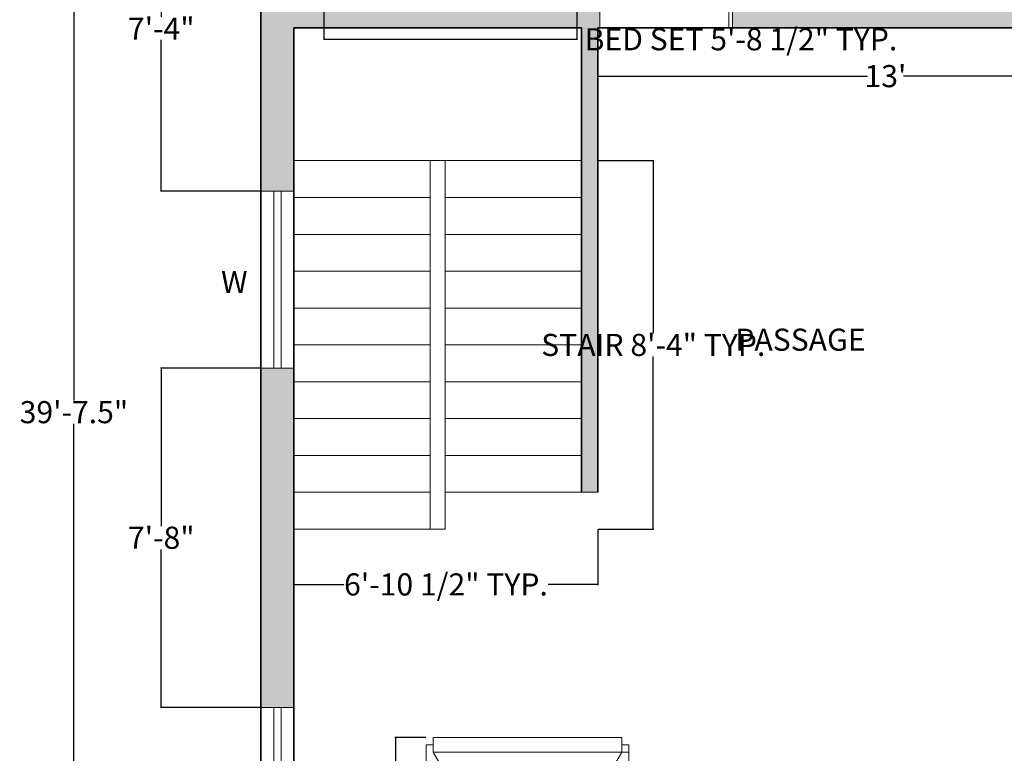
# Model space of a CAD drawing. Units: inches. Extents: x 302 to 1258, y 831 to 1373.
# Tile 8 of 13: x 781 to 1048, y 1012 to 1211. Entities that reach past the tile are written whole.
import ezdxf

# ---------------------------------------------------------------- set-up
doc = ezdxf.new("R2010")
doc.units = ezdxf.units.IN
doc.header["$MEASUREMENT"] = 0
for name, color, linetype, lineweight in [('A-ANNO-DIMS', 2, 'Continuous', 18), ('A-ANNO-TEXT', 7, 'Continuous', 18), ('A-AREA-IDEN', 7, 'Continuous', 18), ('A-DOOR', 3, 'Continuous', 18), ('A-FLOR-STRS', 7, 'Continuous', 18), ('A-FURN', 8, 'Continuous', 18), ('A-GLAZ', 4, 'Continuous', 18), ('A-WALL', 7, 'Continuous', 35), ('A-WALL-PATT', 251, 'Continuous', 13)]:
    doc.layers.add(name, color=color, linetype=linetype, lineweight=lineweight)
doc.styles.get("Standard").update_dxf_attribs({"font": 'arial.ttf'})
doc.dimstyles.get("Standard").update_dxf_attribs({"dimtxt": 6, "dimasz": 0.18, "dimexe": 0.18, "dimexo": 0.0625, "dimgap": 0.09, "dimtad": 0, "dimtih": 1, "dimtoh": 1, "dimdec": 1, "dimzin": 0, "dimdsep": 46, "dimlunit": 3, "dimtxsty": 'Standard', "dimcen": 0.09, "dimadec": 0, "dimazin": 0, "dimtfac": 1, "dimtdec": 1, "dimtofl": 0, "dimtmove": 0, "dimatfit": 3, "dimfxl": 1, "dimtolj": 1, "dimtzin": 0, "dimarcsym": 0})

# ---------------------------------------------------------------- blocks, each defined once
blk = doc.blocks.new('*D30')
at = {"layer": 'A-ANNO-DIMS', "color": 0, "lineweight": -2, "transparency": 16777216}
for p, q in [((937.62, 1208.76), (937.62, 1195.58)), ((1093.62, 1208.76), (1093.62, 1195.58)), ((937.8, 1195.76), (1010.72, 1195.76)), ((1093.44, 1195.76), (1020.52, 1195.76))]:
    blk.add_line(p, q, dxfattribs=at)
at = {"layer": 'A-ANNO-DIMS', "color": 0, "transparency": 16777216}
for points in [[(937.8, 1195.79), (937.8, 1195.73), (937.62, 1195.76)], [(1093.44, 1195.79), (1093.44, 1195.73), (1093.62, 1195.76)]]:
    blk.add_solid(points, dxfattribs=at)
at = {"layer": 'Defpoints', "color": 0, "transparency": 16777216}
for p in [(937.62, 1208.82), (1093.62, 1208.82), (1093.62, 1195.76)]:
    blk.add_point(p, dxfattribs=at)
at = {"layer": 'A-ANNO-DIMS', "color": 0, "transparency": 16777216, "insert": (1015.62, 1195.76), "char_height": 6, "attachment_point": 5}
blk.add_mtext("\\A1;13'", dxfattribs=at)
blk = doc.blocks.new('*D34')
at = {"layer": 'A-ANNO-DIMS', "color": 0, "lineweight": -2, "transparency": 16777216}
for p, q in [((846.06, 1342.32), (795.24, 1342.32)), ((795.42, 1342.14), (795.42, 1107.72)), ((795.42, 867), (795.42, 1101.41)), ((846.06, 866.82), (795.24, 866.82))]:
    blk.add_line(p, q, dxfattribs=at)
at = {"layer": 'A-ANNO-DIMS', "color": 0, "transparency": 16777216}
for points in [[(795.39, 1342.14), (795.45, 1342.14), (795.42, 1342.32)], [(795.39, 867), (795.45, 867), (795.42, 866.82)]]:
    blk.add_solid(points, dxfattribs=at)
at = {"layer": 'Defpoints', "color": 0, "transparency": 16777216}
for p in [(846.12, 1342.32), (795.42, 866.82), (846.12, 866.82)]:
    blk.add_point(p, dxfattribs=at)
at = {"layer": 'A-ANNO-DIMS', "color": 0, "transparency": 16777216, "insert": (795.42, 1104.57), "char_height": 6, "attachment_point": 5}
blk.add_mtext('\\A1;39\'-7.5"', dxfattribs=at)
blk = doc.blocks.new('SOFA-3-SEAT')
for p, q in [((1.96, 55.04), (22.23, 55.04)), ((1.96, 55.04), (1.96, 53.08)), ((3.92, 55.04), (3.92, 1.96)), ((22.23, 51.12), (22.23, 55.04)), ((0, 53.08), (0, 1.96)), ((3.92, 53.08), (0, 53.08)), ((3.92, 53.08), (7.85, 50.88)), ((7.54, 51.12), (22.23, 51.12)), ((21.57, 50.87), (7.85, 50.87)), ((21.57, 35.3), (7.85, 35.3)), ((21.57, 19.74), (7.85, 19.74)), ((7.85, 4.17), (3.92, 1.96)), ((7.28, 3.92), (22.23, 3.92)), ((22.23, 3.92), (22.23, 0)), ((3.92, 1.96), (0, 1.96)), ((1.96, 1.96), (1.96, 0)), ((1.96, 0), (22.23, 0))]:
    blk.add_line(p, q)
blk.add_lwpolyline([(7.85, 50.88), (7.85, 4.17), (21.57, 4.17), (21.57, 50.87)])
blk = doc.blocks.new('WINDOW-48IN')
for p, q in [((0, 0), (0, 9)), ((0, 9), (48, 9)), ((48, 9), (48, 0)), ((0, 5.5), (48, 5.5)), ((48, 3.5), (0, 3.5)), ((48, 0), (0, 0))]:
    blk.add_line(p, q)
blk = doc.blocks.new('DOOR-36IN-BEDROOM')
for p, q in [((35, 36), (35, 0)), ((36, 0), (36, 36)), ((36, 36), (36, 0)), ((0, 0), (0, 4.5)), ((36, 0), (0, 0)), ((37, 0), (36, 0))]:
    blk.add_line(p, q)
blk.add_arc((36, -0.32), 36.32, 90, 172.3719)
blk = doc.blocks.new('STAIR-RETURN-RUNS')
for p, q in [((0, 100), (78, 100)), ((37, 100), (37, 0)), ((41, 100), (41, 0)), ((0, 90), (37, 90)), ((41, 90), (78, 90)), ((0, 80), (37, 80)), ((41, 80), (78, 80)), ((0, 70), (37, 70)), ((41, 70), (78, 70)), ((0, 60), (37, 60)), ((41, 60), (78, 60)), ((0, 50), (37, 50)), ((41, 50), (78, 50)), ((0, 40), (37, 40)), ((41, 40), (78, 40)), ((0, 30), (37, 30)), ((41, 30), (78, 30)), ((0, 20), (37, 20)), ((41, 20), (78, 20)), ((0, 10), (37, 10)), ((41, 10), (82.5, 10)), ((0, 0), (41, 0))]:
    blk.add_line(p, q)
blk = doc.blocks.new('*D48')
at = {"layer": 'A-ANNO-DIMS', "color": 0, "lineweight": -2, "transparency": 16777216}
for p, q in [((890.9, 1016.24), (882.53, 1016.24)), ((882.71, 1016.06), (882.71, 1008.28)), ((882.71, 994.19), (882.71, 1001.97)), ((890.9, 994.01), (882.53, 994.01))]:
    blk.add_line(p, q, dxfattribs=at)
at = {"layer": 'A-ANNO-DIMS', "color": 0, "transparency": 16777216}
for points in [[(882.68, 1016.06), (882.74, 1016.06), (882.71, 1016.24)], [(882.68, 994.19), (882.74, 994.19), (882.71, 994.01)]]:
    blk.add_solid(points, dxfattribs=at)
at = {"layer": 'Defpoints', "color": 0, "transparency": 16777216}
for p in [(890.97, 1016.24), (882.71, 994.01), (890.97, 994.01)]:
    blk.add_point(p, dxfattribs=at)
at = {"layer": 'A-ANNO-DIMS', "color": 0, "transparency": 16777216, "insert": (882.71, 1005.12), "char_height": 6, "attachment_point": 5}
blk.add_mtext('\\A1;1\'-10" TYP.', dxfattribs=at)
blk = doc.blocks.new('*D51')
at = {"layer": 'A-ANNO-DIMS', "color": 0, "lineweight": -2, "transparency": 16777216}
for p, q in [((863.2, 1216), (863.2, 1205.58)), ((931.91, 1216), (931.91, 1205.58)), ((863.38, 1205.76), (931.73, 1205.76)), ((931.91, 1205.76), (932.09, 1205.76))]:
    blk.add_line(p, q, dxfattribs=at)
at = {"layer": 'A-ANNO-DIMS', "color": 0, "transparency": 16777216}
for points in [[(863.38, 1205.79), (863.38, 1205.73), (863.2, 1205.76)], [(931.73, 1205.79), (931.73, 1205.73), (931.91, 1205.76)]]:
    blk.add_solid(points, dxfattribs=at)
at = {"layer": 'Defpoints', "color": 0, "transparency": 16777216}
for p in [(863.2, 1216.06), (931.91, 1216.06), (931.91, 1205.76)]:
    blk.add_point(p, dxfattribs=at)
at = {"layer": 'A-ANNO-DIMS', "color": 0, "transparency": 16777216, "insert": (976.42, 1205.76), "char_height": 6, "attachment_point": 5}
blk.add_mtext('\\A1;BED SET 5\'-8 1/2" TYP.', dxfattribs=at)
blk = doc.blocks.new('*D63')
at = {"layer": 'A-ANNO-DIMS', "color": 0, "lineweight": -2, "transparency": 16777216}
for p, q in [((937.68, 1172.82), (952.8, 1172.82)), ((952.62, 1172.64), (952.62, 1126.01)), ((952.62, 1073), (952.62, 1119.63)), ((937.68, 1072.82), (952.8, 1072.82))]:
    blk.add_line(p, q, dxfattribs=at)
at = {"layer": 'A-ANNO-DIMS', "color": 0, "transparency": 16777216}
for points in [[(952.59, 1172.64), (952.65, 1172.64), (952.62, 1172.82)], [(952.59, 1073), (952.65, 1073), (952.62, 1072.82)]]:
    blk.add_solid(points, dxfattribs=at)
at = {"layer": 'Defpoints', "color": 0, "transparency": 16777216}
for p in [(937.62, 1172.82), (952.62, 1172.82), (937.62, 1072.82)]:
    blk.add_point(p, dxfattribs=at)
at = {"layer": 'A-ANNO-DIMS', "color": 0, "transparency": 16777216, "insert": (952.62, 1122.82), "char_height": 6, "attachment_point": 5}
blk.add_mtext('\\A1;STAIR 8\'-4" TYP.', dxfattribs=at)
blk = doc.blocks.new('*D64')
at = {"layer": 'A-ANNO-DIMS', "color": 0, "lineweight": -2, "transparency": 16777216}
for p, q in [((855.12, 1072.76), (855.12, 1057.64)), ((937.62, 1072.76), (937.62, 1057.64)), ((855.3, 1057.82), (868.66, 1057.82)), ((937.44, 1057.82), (924.09, 1057.82))]:
    blk.add_line(p, q, dxfattribs=at)
at = {"layer": 'A-ANNO-DIMS', "color": 0, "transparency": 16777216}
for points in [[(855.3, 1057.85), (855.3, 1057.79), (855.12, 1057.82)], [(937.44, 1057.85), (937.44, 1057.79), (937.62, 1057.82)]]:
    blk.add_solid(points, dxfattribs=at)
at = {"layer": 'Defpoints', "color": 0, "transparency": 16777216}
for p in [(855.12, 1072.82), (937.62, 1072.82), (937.62, 1057.82)]:
    blk.add_point(p, dxfattribs=at)
at = {"layer": 'A-ANNO-DIMS', "color": 0, "transparency": 16777216, "insert": (896.37, 1057.82), "char_height": 6, "attachment_point": 5}
blk.add_mtext('\\A1;6\'-10 1/2" TYP.', dxfattribs=at)
blk = doc.blocks.new('*D88')
at = {"layer": 'A-ANNO-DIMS', "color": 0, "lineweight": -2, "transparency": 16777216}
for p, q in [((846.05954, 1252.758966), (818.94204, 1252.758966)), ((819.12204, 1252.578966), (819.12204, 1211.744211)), ((819.12204, 1164.729456), (819.12204, 1205.564211)), ((846.05954, 1164.549456), (818.94204, 1164.549456))]:
    blk.add_line(p, q, dxfattribs=at)
at = {"layer": 'A-ANNO-DIMS', "color": 0, "transparency": 16777216}
for points in [[(819.09204, 1252.578966), (819.15204, 1252.578966), (819.12204, 1252.758966)], [(819.09204, 1164.729456), (819.15204, 1164.729456), (819.12204, 1164.549456)]]:
    blk.add_solid(points, dxfattribs=at)
at = {"layer": 'Defpoints', "color": 0, "transparency": 16777216}
for p in [(846.12204, 1252.758966), (819.12204, 1164.549456), (846.12204, 1164.549456)]:
    blk.add_point(p, dxfattribs=at)
at = {"layer": 'A-ANNO-DIMS', "color": 0, "transparency": 16777216, "insert": (819.12204, 1208.654211), "char_height": 6, "attachment_point": 5}
blk.add_mtext('\\A1;7\'-4"', dxfattribs=at)
blk = doc.blocks.new('*D89')
at = {"layer": 'A-ANNO-DIMS', "color": 0, "lineweight": -2, "transparency": 16777216}
for p, q in [((846.06, 1116.55), (818.94, 1116.55)), ((819.12, 1116.37), (819.12, 1073.65)), ((819.12, 1024.62), (819.12, 1067.34)), ((846.06, 1024.44), (818.94, 1024.44))]:
    blk.add_line(p, q, dxfattribs=at)
at = {"layer": 'A-ANNO-DIMS', "color": 0, "transparency": 16777216}
for points in [[(819.09, 1116.37), (819.15, 1116.37), (819.12, 1116.55)], [(819.09, 1024.62), (819.15, 1024.62), (819.12, 1024.44)]]:
    blk.add_solid(points, dxfattribs=at)
at = {"layer": 'Defpoints', "color": 0, "transparency": 16777216}
for p in [(846.12, 1116.55), (819.12, 1024.44), (846.12, 1024.44)]:
    blk.add_point(p, dxfattribs=at)
at = {"layer": 'A-ANNO-DIMS', "color": 0, "transparency": 16777216, "insert": (819.12, 1070.49), "char_height": 6, "attachment_point": 5}
blk.add_mtext('\\A1;7\'-8"', dxfattribs=at)

msp = doc.modelspace()

# ---------------------------------------------------------------- hatches: boundary and pattern name
at = {"layer": 'A-WALL-PATT'}
h = msp.add_hatch(color=256, dxfattribs=at)
h.dxf.hatch_style = 1
h.paths.add_polyline_path([(1003.23, 1342.32), (934.03, 1342.32), (934.03, 1333.32), (975.12, 1333.32), (975.12, 1330.32), (979.62, 1330.32), (979.62, 1333.32), (1003.23, 1333.32)])
h.paths.add_polyline_path([(1203.12, 1342.32), (1027.23, 1342.32), (1027.23, 1333.32), (1045.62, 1333.32), (1045.62, 1213.32), (979.62, 1213.32), (979.62, 1306.32), (975.12, 1306.32), (975.12, 1213.32), (974.12, 1213.32), (974.12, 1208.82), (975.12, 1208.82), (1051.12, 1208.82), (1051.12, 1213.32), (1050.12, 1213.32), (1050.12, 1333.32), (1194.12, 1333.32), (1194.12, 1302.71), (1203.12, 1302.71)])
h.paths.add_polyline_path([(855.12, 1333.32), (886.03, 1333.32), (886.03, 1342.32), (846.12, 1342.32), (846.12, 1300.76), (855.12, 1300.76)])
h.paths.add_polyline_path([(938.12, 1213.32), (855.12, 1213.32), (855.12, 1252.76), (846.12, 1252.76), (846.12, 1164.55), (855.12, 1164.55), (855.12, 1208.82), (933.12, 1208.82), (933.12, 1082.82), (937.62, 1082.82), (937.62, 1208.82), (938.12, 1208.82)])
h.paths.add_polyline_path([(855.12, 1116.55), (846.12, 1116.55), (846.12, 1024.44), (855.12, 1024.44)])
h.paths.add_polyline_path([(855.12, 976.44), (846.12, 976.44), (846.12, 944.2), (855.12, 944.2)])

# ---------------------------------------------------------------- linework, layer by layer
at = {"layer": 'A-WALL'}
for p, q in [((846.12, 1342.32), (846.12, 866.82)), ((855.12, 1208.82), (933.12, 1208.82)), ((855.12, 1208.82), (855.12, 875.82)), ((933.12, 1208.82), (933.12, 1082.82)), ((937.62, 1208.82), (1093.62, 1208.82)), ((937.62, 1208.82), (937.62, 1082.82))]:
    msp.add_line(p, q, dxfattribs=at)

# ---------------------------------------------------------------- block references
at = {"layer": 'A-DOOR'}
msp.add_blockref('DOOR-36IN-BEDROOM', (938.12, 1208.82), dxfattribs=at)
at = {"layer": 'A-FLOR-STRS'}
msp.add_blockref('STAIR-RETURN-RUNS', (855.12, 1072.82), dxfattribs=at)
at = {"layer": 'A-FURN', "rotation": 269.9999999999992}
msp.add_blockref('SOFA-3-SEAT', (890.97, 1016.24), dxfattribs=at)
at = {"layer": 'A-GLAZ'}
for p, rotation in [((846.12, 1164.55), 269.9999999999992), ((855.12, 976.44), 89.99999999999999)]:
    msp.add_blockref('WINDOW-48IN', p, dxfattribs=dict(at, rotation=rotation))

# ---------------------------------------------------------------- texts
at = {"layer": 'A-ANNO-TEXT', "insert": (835.34, 1142.88), "char_height": 6, "attachment_point": 1}
msp.add_mtext_dynamic_manual_height_columns('W', width=16.4894, gutter_width=30, heights=[0], dxfattribs=at)
at = {"layer": 'A-AREA-IDEN', "insert": (974.88, 1127.23), "char_height": 6, "attachment_point": 1}
msp.add_mtext_dynamic_manual_height_columns('PASSAGE', width=60.5592, gutter_width=30, heights=[0], dxfattribs=at)

# ---------------------------------------------------------------- dimensions: what is measured, and where the dimension line sits
at = {"layer": 'A-ANNO-DIMS'}
for base, p1, p2, override, picture, middle in [((795.42, 866.82), (846.12, 1342.32), (846.12, 866.82), {"dimclrd": 0, "dimclre": 0, "dimclrt": 0}, '*D34', (795.42, 1104.57)), ((819.12, 1164.55), (846.12, 1252.76), (846.12, 1164.55), {"dimdec": 1, "dimlfac": 1, "dimrnd": 0, "dimzin": 1, "dimdsep": 46, "dimlunit": 4, "dimfrac": 2}, '*D88', (819.12, 1208.65)), ((819.12, 1024.44), (846.12, 1116.55), (846.12, 1024.44), {"dimdec": 1, "dimlfac": 1, "dimrnd": 0, "dimzin": 1, "dimdsep": 46, "dimlunit": 4, "dimfrac": 2}, '*D89', (819.12, 1070.49))]:
    dim = msp.add_linear_dim(base=base, p1=p1, p2=p2, angle=90, dimstyle='Standard', override=override, dxfattribs=at)
    dim.commit()
    dim.dimension.update_dxf_attribs({"geometry": picture, "text_midpoint": middle})
for base, p1, p2, text, picture, middle in [((931.91, 1205.76), (863.2, 1216.06), (931.91, 1216.06), 'BED SET <> TYP.', '*D51', (976.42, 1205.76)), ((937.62, 1057.82), (855.12, 1072.82), (937.62, 1072.82), '<> TYP.', '*D64', (896.37, 1057.82))]:
    dim = msp.add_linear_dim(base=base, p1=p1, p2=p2, text=text, dimstyle='Standard', override={"dimdec": 1, "dimlfac": 1, "dimrnd": 0, "dimzin": 1, "dimdsep": 46, "dimlunit": 4, "dimfrac": 2}, dxfattribs=at)
    dim.commit()
    dim.dimension.update_dxf_attribs({"geometry": picture, "text_midpoint": middle})
dim = msp.add_linear_dim(base=(1093.62, 1195.76), p1=(937.62, 1208.82), p2=(1093.62, 1208.82), dimstyle='Standard', override={"dimclrd": 0, "dimclre": 0, "dimclrt": 0}, dxfattribs=at)
dim.commit()
dim.dimension.update_dxf_attribs({"geometry": '*D30', "text_midpoint": (1015.62, 1195.76)})
for base, p1, p2, angle, text, picture, middle in [((952.62, 1172.82), (937.62, 1072.82), (937.62, 1172.82), 90, 'STAIR <> TYP.', '*D63', (952.62, 1122.82)), ((882.71, 994.01), (890.97, 1016.24), (890.97, 994.01), 270, '<> TYP.', '*D48', (882.71, 1005.12))]:
    dim = msp.add_linear_dim(base=base, p1=p1, p2=p2, angle=angle, text=text, dimstyle='Standard', override={"dimdec": 1, "dimlfac": 1, "dimrnd": 0, "dimzin": 1, "dimdsep": 46, "dimlunit": 4, "dimfrac": 2}, dxfattribs=at)
    dim.commit()
    dim.dimension.update_dxf_attribs({"geometry": picture, "text_midpoint": middle})

doc.saveas('drawing.dxf')
